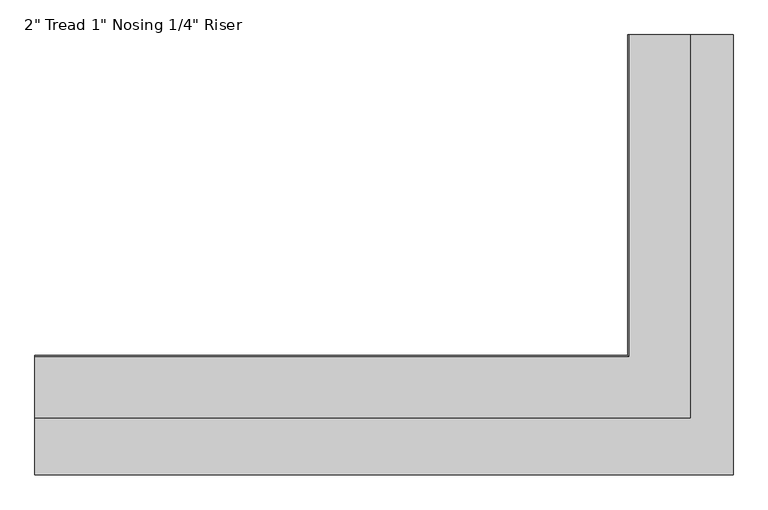
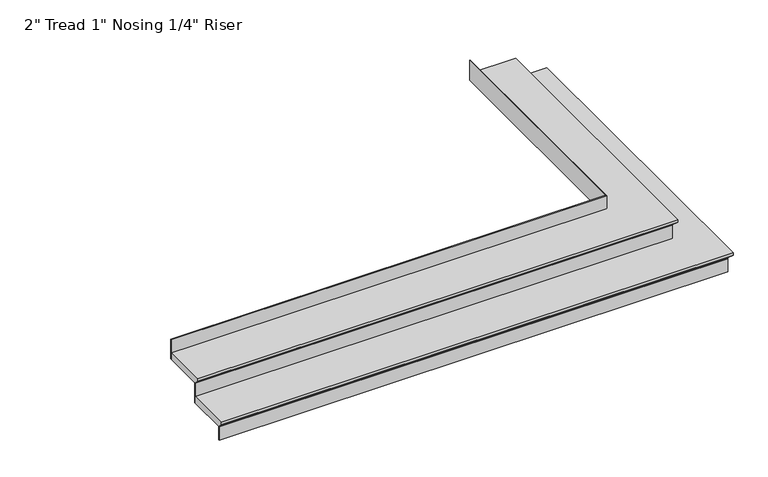
"""IFC4 building model written with IfcOpenShell, lengths in millimetres: stair flight geometry."""

from ifc_helpers import new_model, si_unit, origin, place, context, project, spatial, faceted_brep, source, transform, mapped, element, save


def stair_flight_046a4295(model_context):
    return source(origin(), model_context, "Body", "Brep", [
        faceted_brep([(-1268.7206632, -6237.0948807, 133.35), (-1268.7206632, -6237.0948807, 152.4), (-1268.7206632, -8599.2948807, 152.4), (-1268.7206632, -8599.2948807, 133.35), (-1294.1206632, -6237.0948807, 107.95), (-1294.1206632, -8573.8948807, 107.95), (-5015.2206632, -8599.2948807, 152.4), (-5015.2206632, -8599.2948807, 133.35), (-5015.2206632, -8573.8948807, 107.95), (-1522.7206632, -6237.0948807, 152.4), (-1522.7206632, -8269.0948807, 152.4), (-5015.2206632, -8269.0948807, 152.4), (-5015.2206632, -8573.8948807, 101.6), (-5015.2206632, -8269.0948807, 101.6), (-1522.7206632, -8269.0948807, 101.6), (-1522.7206632, -6237.0948807, 101.6), (-1294.1206632, -6237.0948807, 101.6), (-1294.1206632, -8573.8948807, 101.6)], [[[0, 1, 2, 3]], [[4, 0, 3, 5]], [[3, 2, 6, 7]], [[5, 3, 7, 8]], [[6, 2, 1, 9, 10, 11]], [[12, 13, 14, 15, 16, 17]], [[6, 11, 13, 12, 8, 7]], [[12, 17, 5, 8]], [[17, 16, 4, 5]], [[9, 1, 0, 4, 16, 15]], [[10, 9, 15, 14]], [[11, 10, 14, 13]]]),
        faceted_brep([(-1294.1206632, -6237.0948807, 101.6), (-1294.1206632, -6237.0948807, 0.0), (-1300.4706632, -6237.0948807, 0.0), (-1300.4706632, -6237.0948807, 101.6), (-1294.1206632, -8573.8948807, 101.6), (-1294.1206632, -8573.8948807, 0.0), (-1300.4706632, -8567.5448807, 0.0), (-1300.4706632, -8567.5448807, 101.6), (-5015.2206632, -8573.8948807, 101.6), (-5015.2206632, -8567.5448807, 101.6), (-5015.2206632, -8567.5448807, 0.0), (-5015.2206632, -8573.8948807, 0.0)], [[[0, 1, 2, 3]], [[1, 0, 4, 5]], [[2, 1, 5, 6]], [[3, 2, 6, 7]], [[0, 3, 7, 4]], [[8, 9, 10, 11]], [[5, 4, 8, 11]], [[6, 5, 11, 10]], [[7, 6, 10, 9]], [[4, 7, 9, 8]]]),
        faceted_brep([(-1522.7206632, -6237.0948807, 254.0), (-1522.7206632, -6237.0948807, 101.6), (-1529.0706632, -6237.0948807, 101.6), (-1529.0706632, -6237.0948807, 254.0), (-1522.7206632, -8269.0948807, 254.0), (-1522.7206632, -8269.0948807, 101.6), (-1529.0706632, -8262.7448807, 101.6), (-1529.0706632, -8262.7448807, 254.0), (-5015.2206632, -8269.0948807, 254.0), (-5015.2206632, -8262.7448807, 254.0), (-5015.2206632, -8262.7448807, 101.6), (-5015.2206632, -8269.0948807, 101.6)], [[[0, 1, 2, 3]], [[1, 0, 4, 5]], [[2, 1, 5, 6]], [[3, 2, 6, 7]], [[0, 3, 7, 4]], [[8, 9, 10, 11]], [[5, 4, 8, 11]], [[6, 5, 11, 10]], [[7, 6, 10, 9]], [[4, 7, 9, 8]]]),
        faceted_brep([(-1827.5206632, -6237.0948807, 406.4), (-1827.5206632, -6237.0948807, 254.0), (-1833.8706632, -6237.0948807, 254.0), (-1833.8706632, -6237.0948807, 406.4), (-1827.5206632, -7964.2948807, 406.4), (-1827.5206632, -7964.2948807, 254.0), (-1833.8706632, -7957.9448807, 254.0), (-1833.8706632, -7957.9448807, 406.4), (-5015.2206632, -7964.2948807, 406.4), (-5015.2206632, -7957.9448807, 406.4), (-5015.2206632, -7957.9448807, 254.0), (-5015.2206632, -7964.2948807, 254.0)], [[[0, 1, 2, 3]], [[1, 0, 4, 5]], [[2, 1, 5, 6]], [[3, 2, 6, 7]], [[0, 3, 7, 4]], [[8, 9, 10, 11]], [[5, 4, 8, 11]], [[6, 5, 11, 10]], [[7, 6, 10, 9]], [[4, 7, 9, 8]]]),
        faceted_brep([(-5015.2206632, -8294.4948807, 304.8), (-1497.3206632, -8294.4948807, 304.8), (-1497.3206632, -6237.0948807, 304.8), (-1827.5206632, -6237.0948807, 304.8), (-1827.5206632, -7964.2948807, 304.8), (-5015.2206632, -7964.2948807, 304.8), (-5015.2206632, -8269.0948807, 254.0), (-5015.2206632, -7964.2948807, 254.0), (-1827.5206632, -7964.2948807, 254.0), (-1827.5206632, -6237.0948807, 254.0), (-1522.7206632, -6237.0948807, 254.0), (-1522.7206632, -8269.0948807, 254.0), (-5015.2206632, -8269.0948807, 260.35), (-5015.2206632, -8294.4948807, 285.75), (-1522.7206632, -8269.0948807, 260.35), (-1522.7206632, -6237.0948807, 260.35), (-1497.3206632, -6237.0948807, 285.75), (-1497.3206632, -8294.4948807, 285.75)], [[[0, 1, 2, 3, 4, 5]], [[6, 7, 8, 9, 10, 11]], [[0, 5, 7, 6, 12, 13]], [[6, 11, 14, 12]], [[11, 10, 15, 14]], [[3, 2, 16, 15, 10, 9]], [[4, 3, 9, 8]], [[5, 4, 8, 7]], [[16, 2, 1, 17]], [[15, 16, 17, 14]], [[17, 1, 0, 13]], [[14, 17, 13, 12]]]),
    ])


if __name__ == "__main__":
    model = new_model("IFC4")
    model_context = context("Model", 3, world=origin())
    ifc_project = project(units=[si_unit("LENGTHUNIT", "METRE", prefix="MILLI")], contexts=[model_context])
    site = spatial("IfcSite", under=ifc_project)
    building = spatial("IfcBuilding", under=site)
    placement = place(None, origin())
    stair_flight_shape = stair_flight_046a4295(model_context)
    element("IfcStairFlight", 1, ObjectType="2\" Tread 1\" Nosing 1/4\" Riser", at=placement, inside=building, context=model_context, shape_type="MappedRepresentation", body=[
        mapped(stair_flight_shape, transform((0.0, 0.0, 0.0), x_axis=(1.0, 0.0, 0.0), y_axis=(0.0, 1.0, 0.0), z_axis=(0.0, 0.0, 1.0))),
    ])
    save(model, "model.ifc")
